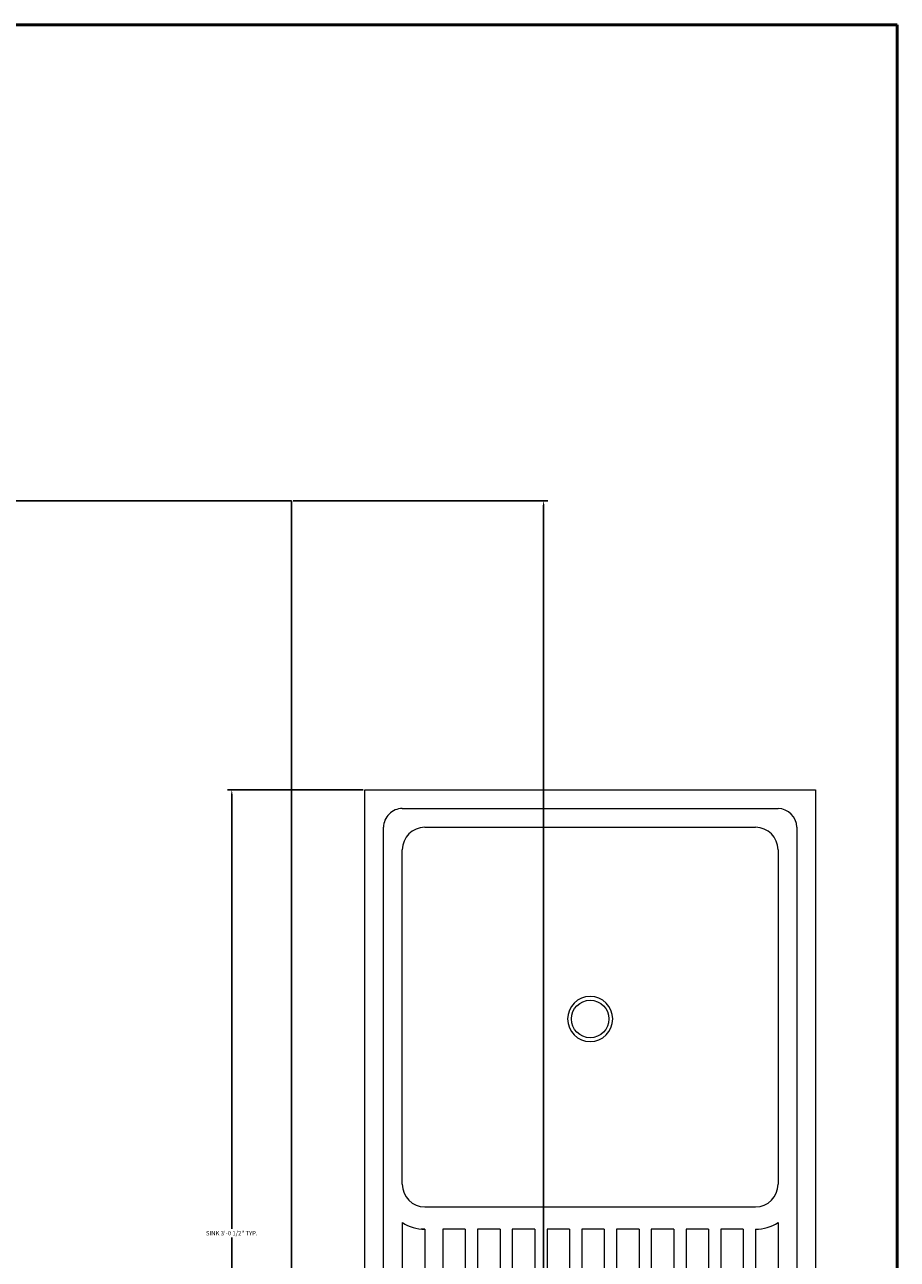
# Model space of a CAD drawing. Units: inches. Extents: x -173 to 545, y -746 to 104.
# Tile 29 of 32: x 225 to 261, y -43 to 8. Entities that reach past the tile are written whole.
import ezdxf

# ---------------------------------------------------------------- set-up
doc = ezdxf.new("R2010")
doc.units = ezdxf.units.IN
doc.header["$MEASUREMENT"] = 0
for name, color, linetype, lineweight in [('A-ANNO-DIMS', 2, 'Continuous', 18), ('A-FLOR-CASE', 9, 'Continuous', 25), ('A-FLOR-FIXT', 8, 'Continuous', 18), ('A-WALL', 7, 'Continuous', 50)]:
    doc.layers.add(name, color=color, linetype=linetype, lineweight=lineweight)
doc.styles.get("Standard").update_dxf_attribs({"font": 'arial.ttf'})
doc.dimstyles.get("Standard").update_dxf_attribs({"dimtxt": 0.18, "dimasz": 0.18, "dimexe": 0.18, "dimexo": 0.0625, "dimgap": 0.09, "dimtad": 0, "dimtih": 1, "dimtoh": 1, "dimdec": 0, "dimzin": 0, "dimdsep": 46, "dimlunit": 3, "dimtxsty": 'Standard', "dimcen": 0.09, "dimadec": 0, "dimazin": 0, "dimtfac": 1, "dimtdec": 0, "dimtofl": 0, "dimtmove": 0, "dimatfit": 3, "dimfxl": 1, "dimtolj": 1, "dimtzin": 0, "dimarcsym": 0})

# ---------------------------------------------------------------- blocks, each defined once
blk = doc.blocks.new('М11 540х1060')
for p, q in [((-1062, 540), (0, 540)), ((-1062, 0), (-1062, 540)), ((0, 540), (0, 0)), ((-1017, 517.5), (-45, 517.5)), ((-1039.5, 45), (-1039.5, 495)), ((-990, 495), (-589.5, 495)), ((-543.7, 495), (-64.8, 495)), ((-22.5, 495), (-22.5, 45)), ((-1017, 72), (-1017, 468)), ((-562.5, 72), (-562.5, 468)), ((-535.7, 468), (-45, 468)), ((-45, 469.5), (-45, 468)), ((-535.7, 453.4), (-45, 453.4)), ((-535.7, 453.4), (-535.7, 426.4)), ((-45, 453.4), (-45, 426.4)), ((-535.7, 426.4), (-45, 426.4)), ((-535.7, 411.8), (-535.7, 384.8)), ((-535.7, 411.8), (-45, 411.8)), ((-45, 411.8), (-45, 384.8)), ((-535.7, 384.8), (-45, 384.8)), ((-535.7, 370.1), (-535.7, 343.1)), ((-535.7, 370.1), (-45, 370.1)), ((-45, 370.1), (-45, 343.1)), ((-535.7, 343.1), (-45, 343.1)), ((-535.7, 328.5), (-535.7, 301.5)), ((-535.7, 328.5), (-45, 328.5)), ((-45, 328.5), (-45, 301.5)), ((-535.7, 301.5), (-45, 301.5)), ((-535.7, 286.9), (-535.7, 259.9)), ((-535.7, 286.9), (-45, 286.9)), ((-45, 286.9), (-45, 259.9)), ((-535.7, 259.9), (-45, 259.9)), ((-535.7, 245.3), (-535.7, 218.3)), ((-535.7, 245.3), (-45, 245.3)), ((-45, 245.3), (-45, 218.3)), ((-535.7, 218.3), (-45, 218.3)), ((-535.7, 203.6), (-535.7, 176.6)), ((-535.7, 203.6), (-45, 203.6)), ((-45, 203.6), (-45, 176.6)), ((-535.7, 176.6), (-45, 176.6)), ((-535.7, 162), (-45, 162)), ((-535.7, 162), (-535.7, 135)), ((-45, 162), (-45, 135)), ((-535.7, 135), (-45, 135)), ((-535.7, 120.4), (-45, 120.4)), ((-535.7, 120.4), (-535.7, 93.4)), ((-45, 120.4), (-45, 93.4)), ((-535.7, 93.4), (-45, 93.4)), ((-535.7, 72), (-45, 72)), ((-535.7, 72), (-535.7, 67.5)), ((-45, 70.5), (-45, 72)), ((-589.5, 45), (-990, 45)), ((-543.7, 45), (-64.8, 45)), ((-45, 22.5), (-1017, 22.5)), ((0, 0), (-1062, 0))]:
    blk.add_line(p, q)
for centre, major_axis, start_param, end_param in [((-1017, 495), (-15.9, 15.9), -0.785398, 0.785398), ((-45, 495), (15.9, 15.9), 5.497787, 7.068583), ((-990, 468), (19.1, 19.1), 0.785398, 2.356194), ((-589.5, 468), (-19.1, 19.1), 3.926991, 5.497787), ((-585.2, 468), (-35, 35), 3.926991, 4.503922), ((-72.3, 468.8), (-19.3, 19.3), 3.899365, 5.250385), ((-787.5, 270), (-19.1, 19.1), 3.926991, 10.210176), ((-787.5, 270), (-15.9, 15.9), 3.926991, 10.210176), ((-990, 72), (-19.1, 19.1), 0.785398, 2.356194), ((-589.5, 72), (19.1, 19.1), 3.926991, 5.497787), ((-585.2, 72), (35, 35), 4.920856, 5.497787), ((-72.3, 71.2), (19.3, 19.3), 4.174393, 5.525413), ((-1017, 45), (15.9, 15.9), 2.356194, 3.926991), ((-45, 45), (-15.9, 15.9), 2.356194, 3.926991)]:
    blk.add_ellipse(centre, major_axis=major_axis, ratio=1, start_param=start_param, end_param=end_param)
blk = doc.blocks.new('COUNTER-L-RETURN')
for p, q in [((66, 69.362), (0, 69.362)), ((66, 0), (66, 69.362))]:
    blk.add_line(p, q)
blk = doc.blocks.new('*D42')
at = {"layer": 'A-ANNO-DIMS', "color": 0, "lineweight": -2, "transparency": 16777216}
for p, q in [((238.763, -23.923), (233.157, -23.923)), ((233.337, -24.103), (233.337, -42.033)), ((233.337, -60.33), (233.337, -42.4)), ((238.763, -60.51), (233.157, -60.51))]:
    blk.add_line(p, q, dxfattribs=at)
at = {"layer": 'A-ANNO-DIMS', "color": 0, "transparency": 16777216}
for points in [[(233.307, -24.103), (233.367, -24.103), (233.337, -23.923)], [(233.307, -60.33), (233.367, -60.33), (233.337, -60.51)]]:
    blk.add_solid(points, dxfattribs=at)
at = {"layer": 'Defpoints', "color": 0, "transparency": 16777216}
for p in [(238.825, -23.923), (233.337, -60.51), (238.825, -60.51)]:
    blk.add_point(p, dxfattribs=at)
at = {"layer": 'A-ANNO-DIMS', "color": 0, "transparency": 16777216, "insert": (233.337, -42.217), "char_height": 0.18, "attachment_point": 5}
blk.add_mtext('\\A1;SINK 3\'-0 1/2" TYP.', dxfattribs=at)
blk = doc.blocks.new('*D76')
at = {"layer": 'A-ANNO-DIMS', "color": 0, "lineweight": -2, "transparency": 16777216}
for p, q in [((235.864, -12), (246.386, -12)), ((246.206, -12.18), (246.206, -46.498)), ((246.206, -81.182), (246.206, -46.864)), ((235.864, -81.362), (246.386, -81.362))]:
    blk.add_line(p, q, dxfattribs=at)
at = {"layer": 'A-ANNO-DIMS', "color": 0, "transparency": 16777216}
for points in [[(246.176, -12.18), (246.236, -12.18), (246.206, -12)], [(246.176, -81.182), (246.236, -81.182), (246.206, -81.362)]]:
    blk.add_solid(points, dxfattribs=at)
at = {"layer": 'Defpoints', "color": 0, "transparency": 16777216}
for p in [(235.801, -12), (246.206, -12), (235.801, -81.362)]:
    blk.add_point(p, dxfattribs=at)
at = {"layer": 'A-ANNO-DIMS', "color": 0, "transparency": 16777216, "insert": (246.206, -46.681), "char_height": 0.18, "attachment_point": 5}
blk.add_mtext('\\A1;COUNTER 5\'-9 1/2" TYP.', dxfattribs=at)

msp = doc.modelspace()

# ---------------------------------------------------------------- linework, layer by layer
at = {"layer": 'A-WALL'}
for p, q in [((169.801, 7.638), (260.801, 7.638)), ((260.801, 7.638), (260.801, -81.362))]:
    msp.add_line(p, q, dxfattribs=at)

# ---------------------------------------------------------------- block references
at = {"layer": 'A-FLOR-CASE'}
msp.add_blockref('COUNTER-L-RETURN', (169.801, -81.362), dxfattribs=at)
at = {"layer": 'A-FLOR-FIXT', "xscale": 0.0344518369672997, "yscale": 0.0344518369672997, "zscale": 0.0344518369672997, "rotation": 270}
msp.add_blockref('М11 540х1060', (238.825, -60.51), dxfattribs=at)

# ---------------------------------------------------------------- dimensions: what is measured, and where the dimension line sits
at = {"layer": 'A-ANNO-DIMS'}
for base, p1, p2, angle, text, picture, middle in [((246.206, -12), (235.801, -81.362), (235.801, -12), 90, 'COUNTER <> TYP.', '*D76', (246.206, -46.681)), ((233.337, -60.51), (238.825, -23.923), (238.825, -60.51), 270, 'SINK <> TYP.', '*D42', (233.337, -42.217))]:
    dim = msp.add_linear_dim(base=base, p1=p1, p2=p2, angle=angle, text=text, dimstyle='Standard', override={"dimdec": 1, "dimlfac": 1, "dimrnd": 0, "dimzin": 1, "dimdsep": 46, "dimlunit": 4, "dimfrac": 2}, dxfattribs=at)
    dim.commit()
    dim.dimension.update_dxf_attribs({"geometry": picture, "text_midpoint": middle})

doc.saveas('drawing.dxf')
